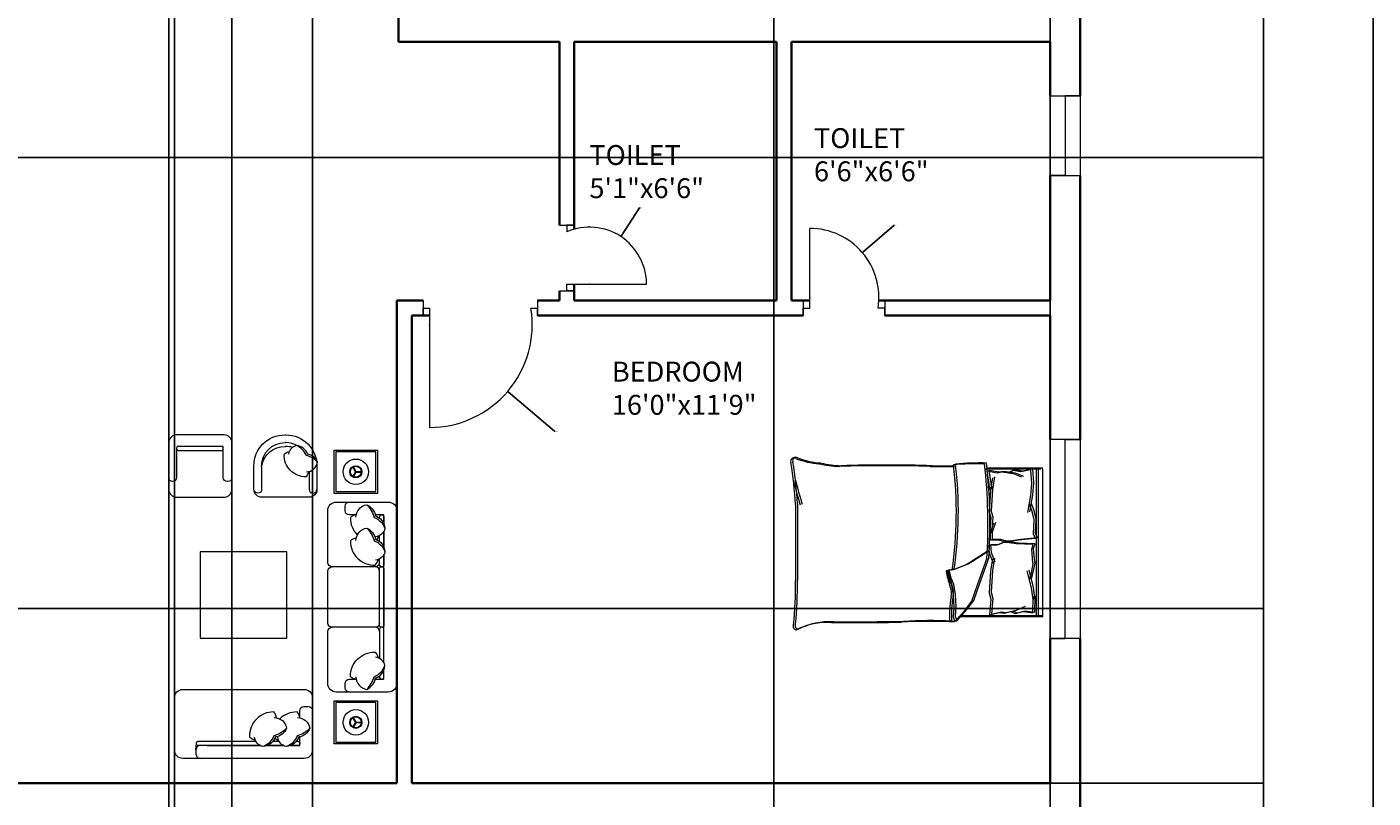
# Model space of a CAD drawing. Units: inches. Extents: x 1902 to 2626, y 1199 to 2408.
# Tile 7 of 9: x 2220 to 2626, y 1817 to 2049. Entities that reach past the tile are written whole.
import ezdxf

# ---------------------------------------------------------------- set-up
doc = ezdxf.new("R2010")
doc.units = ezdxf.units.IN
for name, color, linetype, lineweight in [('A-ANNO-DIMS', 2, 'Continuous', 18), ('A-ANNO-TTLB', 7, 'Continuous', 25), ('A-AREA-IDEN', 7, 'Continuous', 18), ('A-DOOR', 31, 'Continuous', 18), ('A-FURN', 8, 'Continuous', 13), ('A-GLAZ', 181, 'Continuous', 18), ('A-WALL', 7, 'Continuous', 35)]:
    doc.layers.add(name, color=color, linetype=linetype, lineweight=lineweight)
doc.styles.get("Standard").update_dxf_attribs({"font": 'arial.ttf'})
doc.dimstyles.get("Standard").update_dxf_attribs({"dimtxt": 0.18, "dimasz": 0.18, "dimexe": 0.18, "dimexo": 0.0625, "dimgap": 0.09, "dimtad": 0, "dimtih": 1, "dimtoh": 1, "dimdec": 4, "dimzin": 0, "dimdsep": 46, "dimtxsty": 'Standard', "dimcen": 0.09, "dimadec": 0, "dimazin": 0, "dimtfac": 1, "dimtdec": 4, "dimtofl": 0, "dimtmove": 0, "dimatfit": 3, "dimfxl": 1, "dimtolj": 1, "dimtzin": 0, "dimarcsym": 0})

# ---------------------------------------------------------------- blocks, each defined once
blk = doc.blocks.new('BED-DOUBLE')
for p, q in [((25.9, 49.37), (22.87, 45.91)), ((25.9, 49.37), (22.87, 45.91)), ((26.5, 49.58), (23.46, 46.12)), ((26.5, 49.58), (23.46, 46.12)), ((27.53, 49.44), (25.9, 49.37, 3.61)), ((27.53, 49.44), (25.9, 49.37, 3.61)), ((26.48, 47.93), (25.9, 49.37)), ((26.48, 47.93), (25.9, 49.37)), ((28.13, 49.66), (26.5, 49.58, 3.61)), ((28.13, 49.66), (26.5, 49.58, 3.61)), ((27.08, 48.15), (26.5, 49.58)), ((27.08, 48.15), (26.5, 49.58)), ((-0.01, 48.09), (0.59, 48.09)), ((-0.01, 48.09), (-0.01, 3.46)), ((-0.01, 47.87), (24.84, 47.87)), ((-0.01, 47.87), (24.84, 47.87)), ((0.59, 48.09), (25.44, 48.09)), ((0.59, 48.09), (25.44, 48.09)), ((1.43, 3.25), (1.43, 47.87)), ((1.43, 3.25), (1.43, 47.87)), ((2.02, 3.46), (2.02, 48.09)), ((2.02, 3.46), (2.02, 48.09)), ((2.38, 46.8), (2.29, 41.75)), ((2.38, 46.8), (2.29, 41.75)), ((2.38, 46.8), (5.38, 46.44)), ((2.38, 46.8), (5.38, 46.44)), ((2.98, 47.01), (2.89, 41.97)), ((2.98, 47.01), (2.89, 41.96)), ((2.98, 47.01), (5.98, 46.66)), ((2.98, 47.01), (5.98, 46.66)), ((7.7, 46.05), (5.2, 44.94)), ((7.7, 46.05), (5.2, 44.94)), ((5.38, 46.44), (7.78, 47)), ((5.38, 46.44), (7.78, 47)), ((8.3, 46.26), (5.8, 45.16)), ((8.3, 46.26), (5.8, 45.16)), ((5.98, 46.66), (8.38, 47.21)), ((5.98, 46.66), (8.38, 47.21)), ((11.04, 46.8), (7.7, 46.05)), ((11.04, 46.8), (7.7, 46.05)), ((7.78, 47), (8.76, 46.52)), ((7.78, 47), (8.76, 46.52)), ((11.64, 47.01), (8.3, 46.26)), ((11.64, 47.01), (8.3, 46.26)), ((8.38, 47.21), (9.35, 46.73)), ((8.38, 47.21), (9.35, 46.73)), ((12.54, 46.62), (11.04, 46.8)), ((12.54, 46.62), (11.04, 46.8)), ((13.14, 46.83), (11.64, 47.01)), ((13.14, 46.83), (11.64, 47.01)), ((15.47, 47.34), (12.54, 46.62)), ((15.47, 47.34), (12.54, 46.62)), ((16.07, 47.56), (13.14, 46.83)), ((16.07, 47.56), (13.14, 46.83)), ((15.09, 42.55), (15.47, 47.34)), ((15.09, 42.55), (15.47, 47.34)), ((15.69, 42.77), (16.07, 47.56)), ((15.69, 42.77), (16.07, 47.56)), ((22.87, 45.91), (20.84, 43.16)), ((22.87, 45.91), (20.84, 43.16)), ((23.46, 46.12), (21.44, 43.38)), ((23.46, 46.12), (21.44, 43.38)), ((26.19, 45.04), (26.48, 47.93)), ((26.19, 45.04), (26.48, 47.93)), ((26.48, 41.43), (26.19, 45.04)), ((26.48, 41.43), (26.19, 45.04)), ((26.79, 45.26), (27.08, 48.15)), ((26.79, 45.25), (27.08, 48.15)), ((27.08, 41.64), (26.79, 45.26)), ((27.08, 41.64), (26.79, 45.25)), ((2.29, 41.75), (2.37, 42.69)), ((2.29, 41.75), (2.37, 42.69)), ((2.37, 42.69), (2.86, 39.14)), ((2.37, 42.69), (2.86, 39.14)), ((2.89, 41.97), (2.97, 42.9)), ((2.89, 41.96), (2.97, 42.9)), ((2.97, 42.9), (3.46, 39.36)), ((2.97, 42.9), (3.46, 39.35)), ((15.61, 40.72), (15.09, 42.55)), ((15.61, 40.72), (15.09, 42.55)), ((15.21, 34.18), (15.61, 40.72)), ((15.21, 34.18), (15.61, 40.72)), ((16.21, 40.93), (15.69, 42.77)), ((16.21, 40.93), (15.69, 42.77)), ((15.81, 34.39), (16.21, 40.93)), ((15.81, 34.39), (16.21, 40.93)), ((20.84, 43.16), (18.97, 37.96)), ((20.84, 43.16), (18.97, 37.96)), ((21.44, 43.38), (19.56, 38.17)), ((21.44, 43.38), (19.56, 38.17)), ((26.91, 38.25), (26.48, 41.43)), ((26.91, 38.24), (26.48, 41.43)), ((27.51, 38.46), (27.08, 41.64)), ((27.51, 38.46), (27.08, 41.64)), ((2.86, 39.14), (4.12, 34.08)), ((2.86, 39.14), (4.12, 34.08)), ((3.42, 36.61), (2.87, 34.68)), ((3.42, 36.61), (2.87, 34.68)), ((3.46, 39.36), (4.72, 34.29)), ((3.46, 39.35), (4.72, 34.29)), ((4.02, 36.82), (3.47, 34.89)), ((4.02, 36.82), (3.47, 34.89)), ((18.97, 37.96), (16.23, 30.17)), ((18.97, 37.96), (16.23, 30.17)), ((19.56, 38.17), (16.82, 30.38)), ((19.56, 38.17), (16.82, 30.38)), ((27.78, 36.37), (26.91, 38.25)), ((27.78, 36.36), (26.91, 38.24)), ((28.38, 36.58), (27.51, 38.46)), ((28.38, 36.58), (27.51, 38.46)), ((28.96, 34.26), (28.38, 36.58)), ((28.96, 34.26), (28.38, 36.58)), ((73.99, 14.07), (73.99, 37.05)), ((73.99, 14.07), (73.99, 37.05)), ((74.59, 14.28), (74.59, 37.27)), ((74.59, 14.28), (74.59, 37.27)), ((2.87, 34.68), (2.36, 31.94)), ((2.87, 34.68), (2.36, 31.94)), ((3.47, 34.89), (2.96, 32.16)), ((3.47, 34.89), (2.96, 32.16)), ((14.59, 30.41), (15.21, 34.18)), ((14.59, 30.41), (15.21, 34.18)), ((15.18, 30.62), (15.81, 34.39)), ((15.18, 30.62), (15.81, 34.39)), ((22.29, 32.17), (26.48, 33.76)), ((22.29, 32.17), (26.48, 33.76)), ((22.89, 32.38), (27.08, 33.98)), ((22.89, 32.38), (27.08, 33.98)), ((26.48, 33.76), (28.36, 34.05)), ((26.48, 33.76), (28.36, 34.05)), ((27.08, 33.98), (28.96, 34.26)), ((27.08, 33.98), (28.96, 34.26)), ((28.36, 34.05), (27.78, 36.37)), ((28.36, 34.05), (27.78, 36.36)), ((2.36, 31.94), (2.38, 31.64)), ((2.36, 31.94), (2.38, 31.64)), ((2.38, 31.64), (2.78, 27.51)), ((2.38, 31.64), (2.78, 27.51)), ((2.96, 32.16), (2.98, 31.86)), ((2.96, 32.16), (2.98, 31.86)), ((2.98, 31.86), (3.37, 27.72)), ((2.98, 31.86), (3.37, 27.72)), ((15.63, 28.72), (14.43, 31.58)), ((15.63, 28.72), (14.43, 31.58)), ((16.22, 28.93), (15.02, 31.8)), ((16.22, 28.93), (15.02, 31.8)), ((15.77, 26.43), (15.63, 28.72)), ((15.77, 26.43), (15.63, 28.72)), ((16.37, 26.64), (16.22, 28.93)), ((16.37, 26.64), (16.22, 28.93)), ((16.23, 28.26), (22.29, 32.17)), ((16.23, 28.26), (22.29, 32.17)), ((16.82, 28.47), (22.89, 32.38)), ((16.82, 28.47), (22.89, 32.38)), ((1.74, 24.27), (6.74, 24.81)), ((1.74, 24.27), (6.74, 24.81)), ((2.78, 27.51), (2.32, 26.13)), ((2.78, 27.51), (2.32, 26.13)), ((2.32, 26.13), (7.34, 25.9)), ((2.32, 26.13), (7.34, 25.9)), ((2.34, 24.48), (7.33, 25.02)), ((2.34, 24.48), (7.33, 25.02)), ((2.88, 23.13), (2.34, 24.48)), ((2.88, 23.13), (2.34, 24.48)), ((3.37, 27.72), (2.92, 26.34)), ((3.37, 27.72), (2.92, 26.34)), ((2.92, 26.34), (7.94, 26.11)), ((2.92, 26.34), (7.94, 26.11)), ((6.74, 24.81), (9.71, 25.35)), ((6.74, 24.81), (9.71, 25.35)), ((7.33, 25.02), (10.3, 25.56)), ((7.33, 25.02), (10.3, 25.56)), ((7.34, 25.9), (10.34, 25.55)), ((7.34, 25.9), (10.34, 25.55)), ((7.94, 26.11), (10.94, 25.76)), ((7.94, 26.11), (10.94, 25.76)), ((9.71, 25.35), (10.92, 25.35)), ((9.71, 25.35), (10.92, 25.35)), ((10.3, 25.56), (11.52, 25.56)), ((10.3, 25.56), (11.52, 25.56)), ((10.34, 25.55), (11.55, 25.62)), ((10.34, 25.55), (11.55, 25.62)), ((10.92, 25.35), (12.68, 24.81)), ((10.92, 25.35), (12.68, 24.81)), ((10.94, 25.76), (12.15, 25.84)), ((10.94, 25.76), (12.15, 25.84)), ((11.52, 25.56), (13.27, 25.02)), ((11.52, 25.56), (13.27, 25.02)), ((11.55, 25.62), (13.27, 26.27)), ((11.55, 25.62), (13.27, 26.27)), ((12.15, 25.84), (13.87, 26.48)), ((12.15, 25.84), (13.87, 26.48)), ((12.68, 24.81), (15.18, 24.81)), ((12.68, 24.81), (15.18, 24.81)), ((13.27, 26.27), (15.77, 26.43)), ((13.27, 26.27), (15.77, 26.43)), ((13.27, 25.02), (15.78, 25.02)), ((13.27, 25.02), (15.78, 25.02)), ((13.87, 26.48), (16.37, 26.64)), ((13.87, 26.48), (16.37, 26.64)), ((15.18, 24.81), (15.18, 22.51)), ((15.18, 24.81), (15.18, 22.51)), ((15.78, 25.02), (15.78, 22.72)), ((15.78, 25.02), (15.78, 22.72)), ((2.28, 22.92), (1.74, 24.27)), ((2.28, 22.92), (1.74, 24.27)), ((2.15, 18.76), (2.28, 22.92)), ((2.15, 18.76), (2.28, 22.92)), ((2.74, 18.98), (2.88, 23.13)), ((2.74, 18.98), (2.88, 23.13)), ((15.18, 22.51), (14.16, 19.57)), ((15.18, 22.51), (14.16, 19.57)), ((15.78, 22.72), (14.76, 19.79)), ((15.78, 22.72), (14.76, 19.79)), ((15.09, 18.1), (15.47, 22.9)), ((15.09, 18.1), (15.47, 22.9)), ((15.69, 18.32), (16.07, 23.11)), ((15.69, 18.32), (16.07, 23.11)), ((2.15, 18.46), (2.15, 18.76)), ((2.15, 18.46), (2.15, 18.76)), ((2.82, 15.76), (2.15, 18.46)), ((2.82, 15.76), (2.15, 18.46)), ((2.74, 18.68), (2.74, 18.98)), ((2.74, 18.68), (2.74, 18.98)), ((3.42, 15.98), (2.74, 18.68)), ((3.42, 15.98), (2.74, 18.68)), ((3.09, 11.31), (4.04, 16.44)), ((3.09, 11.31), (4.04, 16.44)), ((3.69, 11.52), (4.63, 16.65)), ((3.69, 11.52), (4.63, 16.65)), ((15.61, 16.27), (15.09, 18.1)), ((15.61, 16.27), (15.09, 18.1)), ((15.21, 9.73), (15.61, 16.27)), ((15.21, 9.73), (15.61, 16.27)), ((16.21, 16.49), (15.69, 18.32)), ((16.21, 16.49), (15.69, 18.32)), ((15.81, 9.94), (16.21, 16.49)), ((15.81, 9.94), (16.21, 16.49)), ((3.5, 13.88), (2.82, 15.76)), ((3.5, 13.87), (2.82, 15.76)), ((4.09, 14.09), (3.42, 15.98)), ((4.09, 14.09), (3.42, 15.98)), ((2.82, 7.74), (3.09, 11.31)), ((2.82, 7.74), (3.09, 11.31)), ((3.42, 7.95), (3.69, 11.52)), ((3.42, 7.95), (3.69, 11.52)), ((14.59, 5.96), (15.21, 9.73)), ((14.59, 5.96), (15.21, 9.73)), ((15.18, 6.18), (15.81, 9.94)), ((15.18, 6.18), (15.81, 9.94)), ((15.21, 9.73), (15.51, 8.67)), ((15.21, 9.73), (15.51, 8.67)), ((15.51, 8.67), (16.19, 3.91)), ((15.51, 8.67), (16.19, 3.91)), ((15.81, 9.94), (16.11, 8.88)), ((15.81, 9.94), (16.11, 8.88)), ((16.11, 8.88), (16.78, 4.12)), ((16.11, 8.88), (16.78, 4.12)), ((2.8, 7.64), (2.82, 7.74)), ((2.8, 7.64), (2.82, 7.74)), ((3.11, 3.64), (2.8, 7.64)), ((3.11, 3.64), (2.8, 7.64)), ((3.09, 3.64), (6.06, 4.18)), ((3.09, 3.64), (6.06, 4.18)), ((3.4, 7.86), (3.42, 7.95)), ((3.4, 7.86), (3.42, 7.95)), ((3.71, 3.86), (3.4, 7.86)), ((3.71, 3.86), (3.4, 7.86)), ((3.69, 3.85), (6.66, 4.39)), ((3.69, 3.85), (6.66, 4.39)), ((8.36, 4.72), (5.79, 5.67)), ((8.36, 4.72), (5.79, 5.67)), ((6.06, 4.18), (8.49, 3.78)), ((6.06, 4.18), (8.49, 3.78)), ((8.95, 4.93), (6.39, 5.88)), ((8.95, 4.93), (6.39, 5.88)), ((6.66, 4.39), (9.09, 3.99)), ((6.66, 4.39), (9.09, 3.99)), ((11.73, 4.18), (8.36, 4.72)), ((11.73, 4.18), (8.36, 4.72)), ((8.49, 3.78), (9.44, 4.32)), ((8.49, 3.78), (9.44, 4.32)), ((12.33, 4.39), (8.95, 4.93)), ((12.33, 4.39), (8.95, 4.93)), ((9.09, 3.99), (10.03, 4.53)), ((9.09, 3.99), (10.03, 4.53)), ((13.22, 4.45), (11.73, 4.18)), ((13.22, 4.45), (11.73, 4.18)), ((13.81, 4.66), (12.33, 4.39)), ((13.81, 4.66), (12.33, 4.39)), ((16.19, 3.91), (13.22, 4.45)), ((16.19, 3.91), (13.22, 4.45)), ((16.78, 4.12), (13.81, 4.66)), ((16.78, 4.12), (13.81, 4.66)), ((16.91, 3.25), (-0.01, 3.25)), ((16.91, 3.25), (-0.01, 3.25)), ((17.5, 3.46), (0.59, 3.46)), ((17.5, 3.46), (0.59, 3.46))]:
    blk.add_line(p, q)
for centre, radius, start, end in [((-6.22, 47.93), 33.79, 349.8763, 2.5657), ((-6.22, 47.93), 33.79, 349.8763, 2.5657), ((33.9, 170.19), 120.92, 266.9791, 273.8365), ((33.9, 170.19), 120.92, 266.9791, 273.8365), ((-5.62, 48.14), 33.79, 349.8763, 2.5657), ((-5.62, 48.14), 33.79, 349.8763, 2.5657), ((34.5, 170.41), 120.92, 266.9791, 273.8365), ((34.5, 170.41), 120.92, 266.9791, 273.8365), ((63.32, -4210.02), 4259.62, 90.00217, 90.28689), ((63.32, -4210.02), 4259.62, 90.00217, 90.28689), ((63.92, -4209.8), 4259.62, 90.00217, 90.28689), ((63.92, -4209.8), 4259.62, 90.00217, 90.28689), ((64.11, 71.12), 21.54, 267.4714, 296.4681), ((64.11, 71.12), 21.54, 267.4714, 296.4681), ((64.71, 71.33), 21.54, 267.4714, 296.4681), ((64.71, 71.33), 21.54, 267.4714, 296.4681), ((73.64, 50.81), 1.03, 332.6588, 86.02), ((73.64, 50.81), 1.03, 332.6588, 86.02), ((198.21, 38.43), 124.23, 174.4998, 180.6351), ((198.21, 38.43), 124.23, 174.4998, 180.6351), ((74.24, 51.02), 1.03, 332.6588, 86.02), ((74.24, 51.02), 1.03, 332.6588, 86.02), ((198.8, 38.64), 124.23, 174.4998, 180.6351), ((198.8, 38.64), 124.23, 174.4998, 180.6351), ((32.74, 40.85), 5.81, 168.6608, 203.7384), ((32.74, 40.85), 5.81, 168.6608, 203.7384), ((33.33, 41.06), 5.81, 168.6608, 203.7384), ((33.33, 41.06), 5.81, 168.6608, 203.7384), ((1.38, 29.09), 27.69, 10.6617, 19.8806), ((1.38, 29.09), 27.69, 10.6617, 19.8806), ((1.98, 29.31), 27.69, 10.6617, 19.8806), ((1.98, 29.31), 27.69, 10.6617, 19.8806), ((145.95, 16.58), 120.47, 171.7845, 186.9006), ((145.95, 16.58), 120.47, 171.7845, 186.9006), ((146.55, 16.8), 120.47, 171.7845, 186.9006), ((146.55, 16.8), 120.47, 171.7845, 186.9006), ((28.42, 34.21), 0.172, 250.2464, 1.1377), ((28.42, 34.21), 0.172, 250.2464, 1.1377), ((29.01, 34.43), 0.172, 250.2464, 1.1377), ((29.01, 34.43), 0.172, 250.2464, 1.1377), ((169.99, 19.95), 154.04, 176.0865, 186.7821), ((169.99, 19.95), 154.04, 176.0865, 186.7821), ((170.58, 20.16), 154.04, 176.0865, 186.7821), ((170.58, 20.16), 154.04, 176.0865, 186.7821), ((-22.15, -16.08), 99.41, 13.3832, 17.7053), ((-22.15, -16.08), 99.41, 13.3832, 17.7053), ((-21.55, -15.86), 99.41, 13.3832, 17.7053), ((-21.55, -15.86), 99.41, 13.3832, 17.7053), ((187.53, 20.01), 113.69, 182.9958, 189.4091), ((187.53, 20.01), 113.69, 182.9958, 189.4091), ((188.12, 20.22), 113.69, 182.9958, 189.4091), ((188.12, 20.22), 113.69, 182.9958, 189.4091), ((18.76, 79.52), 77.79, 268.7218, 275.604), ((18.76, 79.52), 77.79, 268.7218, 275.604), ((19.36, 79.74), 77.79, 268.7218, 275.604), ((19.36, 79.74), 77.79, 268.7218, 275.604), ((29.1, -156.22), 158.84, 88.4762, 91.0082), ((29.1, -156.22), 158.84, 88.4762, 91.0082), ((29.7, -156), 158.84, 88.4762, 91.0082), ((29.7, -156.01), 158.84, 88.4762, 91.0082), ((47.26, 452.71), 450.36, 268.2277, 271.7185), ((47.26, 452.71), 450.36, 268.2277, 271.7185), ((47.85, 452.92), 450.36, 268.2277, 271.7185), ((47.85, 452.92), 450.36, 268.2277, 271.7185), ((60.24, -25.11), 27.67, 76.0648, 88.9113), ((60.24, -25.11), 27.67, 76.0648, 88.9113), ((60.83, -24.9), 27.67, 76.0648, 88.9113), ((60.83, -24.9), 27.67, 76.0648, 88.9113), ((65.61, -20.22), 22, 67.9751, 86.652), ((65.61, -20.22), 22, 67.9751, 86.652), ((66.21, -20.01), 22, 67.9751, 86.652), ((66.21, -20.01), 22, 67.9751, 86.652), ((74.43, 1.02), 1.02, 236.1736, 23.4781), ((74.43, 1.02), 1.02, 236.1736, 23.4781), ((75.03, 1.23), 1.02, 236.1736, 23.4781), ((75.03, 1.23), 1.02, 236.1736, 23.4781)]:
    blk.add_arc(centre, radius, start, end)
blk = doc.blocks.new('WINDOW-60-A')
for p, q in [((0, 9), (0, 0)), ((60, 9), (0, 9)), ((60, 4.5), (60, 9)), ((60, 9), (60, 0)), ((0, 0), (0, 4.5)), ((0, 4.5), (60, 4.5)), ((0, 0), (60, 0))]:
    blk.add_line(p, q)
blk = doc.blocks.new('WINDOW-24')
for p, q in [((0, 24), (9, 24)), ((0, 24), (0, 0)), ((9, 24), (4.5, 24)), ((4.5, 24), (4.5, 0)), ((9, 24), (9, 0)), ((4.5, 0), (0, 0)), ((0, 0), (9, 0))]:
    blk.add_line(p, q)
blk = doc.blocks.new('TABLE-END-WITH-LAMP')
for p, q in [((6.59, 6.55), (5.67, 8.14)), ((6.45, 6.47), (5.53, 8.06)), ((6.45, 6.55), (5.53, 4.96)), ((6.59, 6.47), (5.67, 4.88)), ((6.52, 6.59), (8.35, 6.59)), ((6.52, 6.43), (8.35, 6.43))]:
    blk.add_line(p, q)
at = {"ltscale": 0.03}
blk.add_lwpolyline([(0.01, 0), (0.01, 13.02), (13.03, 13.02), (13.03, 0)], close=True, dxfattribs=at)
blk.add_lwpolyline([(0.53, 12.5), (0.53, 0.52), (12.51, 0.52), (12.51, 12.5)], close=True)
for radius in [3.84, 1.84, 1.65]:
    blk.add_circle((6.52, 6.51), radius)
blk = doc.blocks.new('TABLE-COFFEE-SQUARE')
at = {"ltscale": 0.03}
blk.add_lwpolyline([(0, 26.05), (0, 0), (26.05, 0), (26.05, 26.05)], close=True, dxfattribs=at)
blk = doc.blocks.new('*D33')
at = {"layer": 'A-ANNO-DIMS', "color": 0, "lineweight": -2, "transparency": 16777216}
for p, q in [((2537.91, 2289.47), (2593.33, 2289.47)), ((2593.15, 2289.29), (2593.15, 2055.66)), ((2593.15, 1821.65), (2593.15, 2055.29)), ((2528.91, 1821.47), (2593.33, 1821.47))]:
    blk.add_line(p, q, dxfattribs=at)
at = {"layer": 'A-ANNO-DIMS', "color": 0, "transparency": 16777216}
for points in [[(2593.12, 2289.29), (2593.18, 2289.29), (2593.15, 2289.47)], [(2593.12, 1821.65), (2593.18, 1821.65), (2593.15, 1821.47)]]:
    blk.add_solid(points, dxfattribs=at)
at = {"layer": 'Defpoints', "color": 0, "transparency": 16777216}
for p in [(2537.85, 2289.47), (2593.15, 2289.47), (2528.85, 1821.47)]:
    blk.add_point(p, dxfattribs=at)
at = {"layer": 'A-ANNO-DIMS', "color": 0, "transparency": 16777216, "insert": (2593.15, 2055.47), "char_height": 0.18, "attachment_point": 5}
blk.add_mtext('\\A1;468', dxfattribs=at)
blk = doc.blocks.new('*D34')
at = {"layer": 'A-ANNO-DIMS', "color": 0, "lineweight": -2, "transparency": 16777216}
for p, q in [((2528.91, 1821.47), (2593.33, 1821.47)), ((2593.15, 1821.29), (2593.15, 1613.15)), ((2593.15, 1404.65), (2593.15, 1612.79)), ((2537.91, 1404.47), (2593.33, 1404.47))]:
    blk.add_line(p, q, dxfattribs=at)
at = {"layer": 'A-ANNO-DIMS', "color": 0, "transparency": 16777216}
for points in [[(2593.12, 1821.29), (2593.18, 1821.29), (2593.15, 1821.47)], [(2593.12, 1404.65), (2593.18, 1404.65), (2593.15, 1404.47)]]:
    blk.add_solid(points, dxfattribs=at)
at = {"layer": 'Defpoints', "color": 0, "transparency": 16777216}
for p in [(2528.85, 1821.47), (2593.15, 1821.47), (2537.85, 1404.47)]:
    blk.add_point(p, dxfattribs=at)
at = {"layer": 'A-ANNO-DIMS', "color": 0, "transparency": 16777216, "insert": (2593.15, 1612.97), "char_height": 0.18, "attachment_point": 5}
blk.add_mtext('\\A1;417', dxfattribs=at)
blk = doc.blocks.new('*D37')
at = {"layer": 'A-ANNO-DIMS', "color": 0, "lineweight": -2, "transparency": 16777216}
for p, q in [((2445.52, 2280.41), (2445.52, 1198.67)), ((2528.85, 2280.41), (2528.85, 1198.67)), ((2445.7, 1198.85), (2486.79, 1198.85)), ((2528.67, 1198.85), (2487.58, 1198.85))]:
    blk.add_line(p, q, dxfattribs=at)
at = {"layer": 'A-ANNO-DIMS', "color": 0, "transparency": 16777216}
for points in [[(2445.7, 1198.88), (2445.7, 1198.82), (2445.52, 1198.85)], [(2528.67, 1198.88), (2528.67, 1198.82), (2528.85, 1198.85)]]:
    blk.add_solid(points, dxfattribs=at)
at = {"layer": 'Defpoints', "color": 0, "transparency": 16777216}
for p in [(2445.52, 2280.47), (2528.85, 2280.47), (2528.85, 1198.85)]:
    blk.add_point(p, dxfattribs=at)
at = {"layer": 'A-ANNO-DIMS', "color": 0, "transparency": 16777216, "insert": (2487.18, 1198.85), "char_height": 0.18, "attachment_point": 5}
blk.add_mtext('\\A1;83.33', dxfattribs=at)
blk = doc.blocks.new('*D39')
at = {"layer": 'A-ANNO-DIMS', "color": 0, "lineweight": -2, "transparency": 16777216}
for p, q in [((2128.41, 2010.11), (2593.33, 2010.11)), ((2593.15, 2009.93), (2593.15, 1942.29)), ((2593.15, 1874.29), (2593.15, 1941.93)), ((2128.41, 1874.11), (2593.33, 1874.11))]:
    blk.add_line(p, q, dxfattribs=at)
at = {"layer": 'A-ANNO-DIMS', "color": 0, "transparency": 16777216}
for points in [[(2593.12, 2009.93), (2593.18, 2009.93), (2593.15, 2010.11)], [(2593.12, 1874.29), (2593.18, 1874.29), (2593.15, 1874.11)]]:
    blk.add_solid(points, dxfattribs=at)
at = {"layer": 'Defpoints', "color": 0, "transparency": 16777216}
for p in [(2128.35, 2010.11), (2593.15, 2010.11), (2128.35, 1874.11)]:
    blk.add_point(p, dxfattribs=at)
at = {"layer": 'A-ANNO-DIMS', "color": 0, "transparency": 16777216, "insert": (2593.15, 1942.11), "char_height": 0.18, "attachment_point": 5}
blk.add_mtext('\\A1;136', dxfattribs=at)
blk = doc.blocks.new('*D41')
at = {"layer": 'A-ANNO-DIMS', "color": 0, "lineweight": -2, "transparency": 16777216}
for p, q in [((2264.77, 1723.47), (2264.77, 2377.95)), ((2264.95, 2377.77), (2285.22, 2377.77)), ((2306.27, 2377.77), (2286.01, 2377.77)), ((2306.45, 1723.47), (2306.45, 2377.95))]:
    blk.add_line(p, q, dxfattribs=at)
at = {"layer": 'A-ANNO-DIMS', "color": 0, "transparency": 16777216}
for points in [[(2264.95, 2377.8), (2264.95, 2377.74), (2264.77, 2377.77)], [(2306.27, 2377.8), (2306.27, 2377.74), (2306.45, 2377.77)]]:
    blk.add_solid(points, dxfattribs=at)
at = {"layer": 'Defpoints', "color": 0, "transparency": 16777216}
for p in [(2306.45, 2377.77), (2264.77, 1723.41), (2306.45, 1723.41)]:
    blk.add_point(p, dxfattribs=at)
at = {"layer": 'A-ANNO-DIMS', "color": 0, "transparency": 16777216, "insert": (2285.61, 2377.77), "char_height": 0.18, "attachment_point": 5}
blk.add_mtext('\\A1;41.68', dxfattribs=at)
blk = doc.blocks.new('*D43')
at = {"layer": 'A-ANNO-DIMS', "color": 0, "lineweight": -2, "transparency": 16777216}
for p, q in [((2263.07, 1800.47), (2263.07, 2377.95)), ((2263.25, 2377.77), (2272.13, 2377.77)), ((2281.92, 2377.77), (2273.04, 2377.77)), ((2282.1, 1800.47), (2282.1, 2377.95))]:
    blk.add_line(p, q, dxfattribs=at)
at = {"layer": 'A-ANNO-DIMS', "color": 0, "transparency": 16777216}
for points in [[(2263.25, 2377.8), (2263.25, 2377.74), (2263.07, 2377.77)], [(2281.92, 2377.8), (2281.92, 2377.74), (2282.1, 2377.77)]]:
    blk.add_solid(points, dxfattribs=at)
at = {"layer": 'Defpoints', "color": 0, "transparency": 16777216}
for p in [(2282.1, 2377.77), (2263.07, 1800.41), (2282.1, 1800.41)]:
    blk.add_point(p, dxfattribs=at)
at = {"layer": 'A-ANNO-DIMS', "color": 0, "transparency": 16777216, "insert": (2272.58, 2377.77), "char_height": 0.18, "attachment_point": 5}
blk.add_mtext('\\A1;19.024', dxfattribs=at)
blk = doc.blocks.new('*D45')
at = {"layer": 'A-ANNO-DIMS', "color": 0, "lineweight": -2, "transparency": 16777216}
for p, q in [((2341.64, 1959.66), (2341.82, 1959.66)), ((2341.73, 1959.57), (2341.73, 1959.75)), ((2379.41, 1927.56), (2365.42, 1939.48)), ((2379.59, 1927.56), (2379.41, 1927.56))]:
    blk.add_line(p, q, dxfattribs=at)
at = {"layer": 'A-ANNO-DIMS', "color": 0, "transparency": 16777216}
blk.add_solid([(2365.44, 1939.51), (2365.4, 1939.46), (2365.28, 1939.6)], dxfattribs=at)
at = {"layer": 'Defpoints', "color": 0, "transparency": 16777216}
for p in [(2341.73, 1959.66), (2365.28, 1939.6)]:
    blk.add_point(p, dxfattribs=at)
at = {"layer": 'A-ANNO-DIMS', "color": 0, "transparency": 16777216, "insert": (2380.07, 1927.56), "char_height": 0.18, "attachment_point": 5}
blk.add_mtext('\\A1;R30.94', dxfattribs=at)
blk = doc.blocks.new('*D55')
at = {"layer": 'A-ANNO-DIMS', "color": 0, "lineweight": -2, "transparency": 16777216}
for p, q in [((2481.65, 1989.57), (2472.31, 1981.57)), ((2481.83, 1989.57), (2481.65, 1989.57)), ((2456.28, 1967.92), (2456.46, 1967.92)), ((2456.37, 1967.83), (2456.37, 1968.01))]:
    blk.add_line(p, q, dxfattribs=at)
at = {"layer": 'A-ANNO-DIMS', "color": 0, "transparency": 16777216}
blk.add_solid([(2472.29, 1981.59), (2472.33, 1981.55), (2472.17, 1981.45)], dxfattribs=at)
at = {"layer": 'Defpoints', "color": 0, "transparency": 16777216}
for p in [(2472.17, 1981.45), (2456.37, 1967.92)]:
    blk.add_point(p, dxfattribs=at)
at = {"layer": 'A-ANNO-DIMS', "color": 0, "transparency": 16777216, "insert": (2482.24, 1989.57), "char_height": 0.18, "attachment_point": 5}
blk.add_mtext('\\A1;R20.8', dxfattribs=at)
blk = doc.blocks.new('*D60')
at = {"layer": 'A-ANNO-DIMS', "color": 0, "lineweight": -2, "transparency": 16777216}
for p, q in [((2405, 1994.89), (2399.45, 1986.43)), ((2405.18, 1994.89), (2405, 1994.89)), ((2389.85, 1971.93), (2390.03, 1971.93)), ((2389.94, 1971.84), (2389.94, 1972.02))]:
    blk.add_line(p, q, dxfattribs=at)
at = {"layer": 'A-ANNO-DIMS', "color": 0, "transparency": 16777216}
blk.add_solid([(2399.42, 1986.45), (2399.47, 1986.41), (2399.35, 1986.28)], dxfattribs=at)
at = {"layer": 'Defpoints', "color": 0, "transparency": 16777216}
for p in [(2399.35, 1986.28), (2389.94, 1971.93)]:
    blk.add_point(p, dxfattribs=at)
at = {"layer": 'A-ANNO-DIMS', "color": 0, "transparency": 16777216, "insert": (2405.73, 1994.89), "char_height": 0.18, "attachment_point": 5}
blk.add_mtext('\\A1;R17.163', dxfattribs=at)

msp = doc.modelspace()

# ---------------------------------------------------------------- linework, layer by layer
at = {"layer": 'A-ANNO-TTLB'}
msp.add_lwpolyline([(1901.6928, 2408.1473), (2626.1646, 2408.1473), (2626.1646, 1206.3103), (1901.6928, 1206.3103)], close=True, dxfattribs=at)
at = {"layer": 'A-DOOR'}
for p, q in [((2380.8507, 1989.6712), (2385.3507, 1989.6712)), ((2385.3507, 1989.6712), (2383.1007, 1989.6712)), ((2383.1007, 1989.6712), (2383.1007, 1987.6712)), ((2456.3714, 1964.7233), (2456.3714, 1988.7233)), ((2380.8507, 1969.9292), (2385.3507, 1969.9292)), ((2383.1007, 1969.9292), (2383.1007, 1971.9292)), ((2383.1007, 1971.9292), (2407.1007, 1971.9292)), ((2385.3507, 1969.9292), (2383.1007, 1969.9292)), ((2339.7263, 1966.9733), (2339.7263, 1962.4733)), ((2339.7263, 1962.4733), (2339.7263, 1964.7233)), ((2339.7263, 1964.7233), (2341.7263, 1964.7233)), ((2341.7263, 1964.7233), (2341.7263, 1940.7233)), ((2374.2725, 1964.5854), (2372.2725, 1964.5854)), ((2374.2725, 1966.9733), (2374.2725, 1963.4615)), ((2374.2725, 1962.4733), (2374.2725, 1964.5854)), ((2454.3714, 1966.9733), (2454.3714, 1962.4733)), ((2454.3714, 1962.4733), (2454.3714, 1964.7233)), ((2454.3714, 1964.7233), (2454.3714, 1964.7233)), ((2454.3714, 1964.7233), (2456.3714, 1964.7233)), ((2478.9238, 1964.7233), (2476.9238, 1964.7233)), ((2478.9238, 1966.9733), (2478.9238, 1962.4733)), ((2478.9238, 1962.4733), (2478.9238, 1964.7233)), ((2374.2725, 1963.4615), (2374.2725, 1962.4733)), ((2341.7263, 1940.7233), (2341.7263, 1928.7233))]:
    msp.add_line(p, q, dxfattribs=at)
for centre, radius, start, end in [((2389.938, 1971.9292), 17.1627, 360, 113.476935), ((2456.3714, 1967.9233), 20.8, 351.150212, 90), ((2341.7263, 1959.6635), 30.9402, 270, 9.153494)]:
    msp.add_arc(centre, radius, start, end, dxfattribs=at)
at = {"layer": 'A-FURN'}
msp.add_line((2271.2864, 1831.5107), (2271.4129, 1833.4644), dxfattribs=at)
at = {"layer": 'A-FURN', "ltscale": 0.03}
for points in [[(2265.4197, 1926.485), (2265.4197, 1926.485, 0.41421356), (2263.071, 1924.1363), (2263.071, 1910.0441, 0.41421356), (2265.4197, 1907.6955), (2265.4197, 1907.6955), (2279.7467, 1907.6955, 0.41421356), (2282.0954, 1910.0441), (2282.0954, 1924.1363, 0.41421356), (2279.7467, 1926.485)], [(2313.6163, 1848.9269, -0.41421356), (2311.0114, 1851.5318), (2311.0114, 1867.1613, -0.41421356), (2312.3138, 1868.4638, -0.41421356), (2311.0114, 1869.7662), (2311.0114, 1885.3957, -0.41421356), (2312.3138, 1886.6982, -0.41421356), (2311.0114, 1888.0006), (2311.0114, 1903.6301, -0.41421356), (2313.6163, 1906.2351), (2329.2458, 1906.2351, -0.41421356), (2331.8507, 1903.6301), (2331.8507, 1851.5318, -0.41421356), (2329.2458, 1848.9269)], [(2264.7741, 1847.1402, -0.41421356), (2267.379, 1849.7451), (2267.379, 1849.7451, 0.31783725), (2267.379, 1849.7451, -0.41421356), (2267.379, 1849.7451), (2267.379, 1849.7451, 1.18618475), (2267.379, 1849.7451, -0.41421356), (2267.379, 1849.7451), (2303.8478, 1849.7451, -0.41421356), (2306.4528, 1847.1402), (2306.4528, 1831.5107, -0.41421356), (2303.8478, 1828.9058), (2267.379, 1828.9058, -0.41421356), (2264.7741, 1831.5107)]]:
    msp.add_lwpolyline(points, format="xyb", close=True, dxfattribs=at)
msp.add_lwpolyline([(2298.2473, 1907.6955), (2291.0838, 1907.6955, -0.41421356), (2288.7351, 1910.0441), (2288.7351, 1917.0902, -0.41421356), (2298.1298, 1926.485), (2298.2473, 1926.485), (2298.3647, 1926.485, -0.41421356), (2307.7595, 1917.0902), (2307.7595, 1910.0441, -0.41421356), (2305.4108, 1907.6955), (2298.2473, 1907.6955)], format="xyb", dxfattribs=at)
at = {"layer": 'A-FURN'}
for points in [[(2291.0838, 1917.0902, -0.41421356), (2298.1298, 1924.1363), (2298.2473, 1924.1363)], [(2301.8623, 1923.207, 0.13059149), (2298.3647, 1924.1363), (2298.2473, 1924.1363)], [(2265.4197, 1922.2574), (2265.4197, 1913.5672, -0.41421356), (2264.2453, 1912.3928), (2264.2453, 1912.3928, -0.41421356), (2263.071, 1913.5672)], [(2275.0876, 1922.962), (2265.8894, 1922.962, 0.41421356), (2265.4197, 1922.4922), (2265.4197, 1922.2574, 0.41421356), (2265.8894, 1921.7876), (2273.9051, 1921.7876, 0.41421356)], [(2273.9051, 1921.7876), (2279.0421, 1921.7876, 0.41421356), (2279.5118, 1922.2574), (2279.5118, 1922.4922, 0.41421356), (2279.0421, 1922.962)], [(2279.0421, 1922.962), (2275.0876, 1922.962, 0.41421356)], [(2291.0838, 1917.0902, -0.37271891), (2298.1298, 1922.962), (2298.2473, 1922.962)], [(2305.1785, 1915.3872, -0.16554063), (2304.452, 1913.8356, -0.42598917), (2297.8566, 1920.563, -0.12152332), (2299.4222, 1921.4903, 7.11546429)], [(2300.3669, 1922.7089, 0.07238424), (2298.3647, 1922.962), (2298.2473, 1922.962)], [(2304.9935, 1920.4548, 0.30666349), (2301.4908, 1923.254, 0.30632997), (2299.2026, 1920.6976, -0.87284716)], [(2307.9516, 1918.2757, 0.14772988), (2304.5193, 1920.2939, 0.21334276), (2301.4908, 1923.254, 0.17866181)], [(2304.5866, 1915.3156, 0.35677236), (2307.9516, 1918.2757, 0.24954205), (2304.9026, 1920.715, -9.61688035)], [(2291.0838, 1917.0903), (2291.0838, 1910.0441, -0.41421356), (2289.9094, 1908.8698), (2289.9094, 1908.8698, -0.41421356), (2288.7351, 1910.0441)], [(2282.0954, 1913.5672, -0.41421356), (2280.921, 1912.3928), (2280.6862, 1912.3928, -0.41421356), (2279.5118, 1913.5672), (2279.5118, 1915.3867)], [(2305.4108, 1915.4437), (2305.4108, 1910.0441, 0.41421356), (2306.5851, 1908.8698), (2306.5851, 1908.8698, 0.41421356), (2307.7595, 1910.0441)], [(2319.5416, 1902.3277), (2317.5236, 1902.3277, -0.41421356), (2316.2212, 1903.6301), (2316.2212, 1904.9326, -0.41421356), (2317.5236, 1906.2351)], [(2319.4628, 1901.6741, -0.35677236), (2322.7458, 1905.4061, -0.24954205), (2325.4513, 1902.0245)], [(2322.7458, 1905.4061, -0.14772988), (2324.9842, 1901.5994, -0.21334276), (2328.2672, 1898.2406)], [(2319.5422, 1902.3305, 0.16554063), (2317.8213, 1901.5248, 0.20023115), (2319.9172, 1896.3545)], [(2325.1626, 1902.1253, -0.30666349), (2328.2672, 1898.2406, -0.30632997), (2325.4319, 1895.7027)], [(2327.9433, 1899.5877), (2327.9433, 1902.3277), (2325.3837, 1902.3277, -0.41435211)], [(2326.6408, 1901.3338), (2326.6408, 1901.8067, -0.41421356), (2327.1618, 1902.3277), (2327.4223, 1902.3277, -0.41421356), (2327.9433, 1901.8067)], [(2327.9433, 1901.8067), (2327.9433, 1899.5877, -0.41446868)], [(2319.4628, 1894.6578, -0.35677236), (2322.7458, 1898.3898, -0.24954205), (2325.4513, 1895.0082)], [(2322.7458, 1898.3898, -0.14772988), (2324.9842, 1894.5831, -0.21334276), (2328.2672, 1891.2243)], [(2325.8019, 1894.8544, 0.07186538), (2326.3111, 1895.9463)], [(2326.6408, 1894.3175), (2326.6408, 1896.1094, -0.41459885)], [(2327.9433, 1897.4209), (2327.9433, 1892.5714, -0.41474665)], [(2319.5422, 1895.3142, 0.16554063), (2317.8213, 1894.5085, 0.42598917), (2325.2827, 1887.1936, 0.12152332), (2326.3111, 1888.93)], [(2325.1626, 1895.109, -0.30666349), (2328.2672, 1891.2243, -0.30632997), (2325.4319, 1888.6865)], [(2326.6408, 1888.0006, -0.41421356), (2325.3384, 1886.6982), (2312.3138, 1886.6982, -0.41732018)], [(2327.9433, 1890.4046), (2327.9433, 1887.2192, -0.41421356), (2327.4223, 1886.6982), (2327.1618, 1886.6982, -0.41421356), (2326.6408, 1887.2192), (2326.6408, 1889.0931, -0.12631336)], [(2326.6408, 1885.3957, 0.41421356), (2325.3384, 1886.6982)], [(2326.6408, 1867.1613, 0.41421356), (2325.3384, 1868.4638), (2312.3138, 1868.4638, 0.4152491)], [(2326.6408, 1869.7662, -0.41421356), (2325.3384, 1868.4638)], [(2327.9433, 1857.7411), (2327.9433, 1867.9428, 0.41421356), (2327.4223, 1868.4638), (2327.1618, 1868.4638, 0.41421356), (2326.6408, 1867.9428), (2326.6408, 1859.0526, 0.41265155)], [(2319.5422, 1852.8315, -0.16554063), (2317.8213, 1853.6372, -0.42598917), (2325.2827, 1860.9521, -0.12152332), (2326.3111, 1859.2156)], [(2325.1626, 1853.0367, 0.30666349), (2328.2672, 1856.9214, 0.30632997), (2325.4319, 1859.4592)], [(2322.7458, 1849.7558, 0.14772988), (2324.9842, 1853.5626, 0.21334276), (2328.2672, 1856.9214)], [(2327.9433, 1853.3553), (2327.9433, 1855.5743, 0.41253535)], [(2317.5236, 1848.9269, -0.41421356), (2316.2212, 1850.2294), (2316.2212, 1851.5318, -0.41421356), (2317.5236, 1852.8343), (2319.5416, 1852.8343)], [(2319.4628, 1853.4879, 0.35677236), (2322.7458, 1849.7558, 0.24954205), (2325.4513, 1853.1374)], [(2326.6408, 1853.8282), (2326.6408, 1853.3553, 0.41421356), (2327.1618, 1852.8343), (2327.4223, 1852.8343, 0.41421356), (2327.9433, 1853.3553)], [(2295.5319, 1841.2143, 0.16554063), (2294.7262, 1842.9352, 0.42598917), (2287.4113, 1835.4738, 0.12152332), (2289.1477, 1834.4454, -7.11546429)], [(2302.5482, 1841.2143, 0.16554063), (2301.7425, 1842.9352, 0.20023115), (2296.5722, 1840.8393, 0.12152332)], [(2302.5454, 1841.2148), (2302.5454, 1843.2328, -0.41421356), (2303.8478, 1844.5353), (2305.1503, 1844.5353, -0.41421356), (2306.4528, 1843.2328)], [(2294.8755, 1841.2937, -0.35677236), (2298.6075, 1838.0107, -0.24954205), (2295.2259, 1835.3052, 9.61688035)], [(2301.8918, 1841.2937, -0.35677236), (2305.6238, 1838.0107, -0.24954205), (2302.2422, 1835.3052, 9.61688035)], [(2295.3267, 1835.5939, -0.30666349), (2291.442, 1832.4893, -0.30632997), (2288.9042, 1835.3246, 0.87284716)], [(2298.6075, 1838.0107, -0.14772988), (2294.8008, 1835.7723, -0.21334276), (2291.442, 1832.4893, -0.17866181)], [(2295.0721, 1834.9546, 0.07186538), (2296.164, 1834.4454, -7.11546429)], [(2302.343, 1835.5939, -0.30666349), (2298.4583, 1832.4893, -0.30632997), (2295.9204, 1835.3246, 0.87284716)], [(2305.6238, 1838.0107, -0.14772988), (2301.8171, 1835.7723, -0.21334276), (2298.4583, 1832.4893, -0.17866181)], [(2299.8054, 1832.8132), (2302.5454, 1832.8132), (2302.5454, 1835.3728, -0.41421356)], [(2274.6068, 1832.8132), (2272.5889, 1832.8132, 0.41421356), (2271.2864, 1831.5107), (2271.2864, 1830.2083, 0.41421356), (2272.5889, 1828.9058)], [(2290.6223, 1832.8132), (2271.9339, 1832.8132, -0.41421356), (2271.4129, 1833.3341), (2271.4129, 1833.5946, -0.41421356), (2271.9339, 1834.1156), (2289.3108, 1834.1156, -0.41421356)], [(2297.6386, 1832.8132), (2292.7891, 1832.8132, -0.41421356)], [(2294.5352, 1834.1156), (2296.3271, 1834.1156, -0.41421356)], [(2302.0244, 1832.8132), (2299.8054, 1832.8132, -0.41421356)], [(2301.5515, 1834.1156), (2302.0244, 1834.1156, -0.41421356), (2302.5454, 1833.5946), (2302.5454, 1833.3341, -0.41421356), (2302.0244, 1832.8132)]]:
    msp.add_lwpolyline(points, format="xyb", dxfattribs=at)
for points in [[(2275.0876, 1922.962), (2265.5371, 1922.962)], [(2279.5118, 1915.3867), (2279.5118, 1922.962), (2275.0876, 1922.962)], [(2327.9433, 1892.5714), (2327.9433, 1897.4209)], [(2327.9433, 1857.7411), (2327.9433, 1890.4046)], [(2325.3837, 1852.8343), (2327.9433, 1852.8343), (2327.9433, 1855.5743)], [(2274.6068, 1832.8132), (2290.6223, 1832.8132)], [(2292.7891, 1832.8132), (2297.6386, 1832.8132)]]:
    msp.add_lwpolyline(points, dxfattribs=at)
msp.add_lwpolyline([(2327.9433, 1886.1772), (2327.9433, 1868.9848, -0.41421356), (2327.4223, 1868.4638), (2327.1618, 1868.4638, -0.41421356), (2326.6408, 1868.9848), (2326.6408, 1886.1772, -0.41421356), (2327.1618, 1886.6982), (2327.4223, 1886.6982, -0.41421356)], format="xyb", close=True, dxfattribs=at)
at = {"layer": 'A-WALL'}
for p, q in [((2332.3507, 2067.5809), (2332.3507, 2044.9733)), ((2537.8507, 2069.0784), (2537.8507, 2028.722)), ((2380.8507, 2044.9733), (2332.3507, 2044.9733)), ((2380.8507, 2044.9733), (2380.8507, 1989.6712)), ((2385.3507, 2044.9733), (2385.3507, 1988.4675)), ((2446.3507, 2044.9733), (2385.3507, 2044.9733)), ((2446.3507, 2044.9733), (2446.3507, 1966.9733)), ((2528.8507, 2044.9733), (2450.8507, 2044.9733)), ((2450.8507, 2044.9733), (2450.8507, 1966.9733)), ((2528.8507, 2044.9733), (2528.8507, 2028.722)), ((2528.8507, 2004.722), (2528.8507, 1966.9733)), ((2537.8507, 2004.722), (2537.8507, 1925.0569)), ((2380.8507, 1969.9292), (2380.8507, 1966.9733)), ((2385.3507, 1971.9292), (2385.3507, 1966.9733)), ((2331.8507, 1966.9733), (2339.7263, 1966.9733)), ((2331.8507, 1966.9733), (2331.8507, 1821.4733)), ((2374.2725, 1966.9733), (2380.8507, 1966.9733)), ((2385.3507, 1966.9733), (2446.3507, 1966.9733)), ((2450.8507, 1966.9733), (2456.3714, 1966.9733)), ((2477.1497, 1966.9733), (2528.8507, 1966.9733)), ((2336.3507, 1962.4733), (2336.3507, 1821.4733)), ((2341.7263, 1962.4733), (2336.3507, 1962.4733)), ((2454.3714, 1962.4733), (2374.2725, 1962.4733)), ((2528.8507, 1962.4733), (2478.9238, 1962.4733)), ((2528.8507, 1962.4733), (2528.8507, 1925.0569)), ((2528.8507, 1865.0569), (2528.8507, 1821.4733)), ((2537.8507, 1865.0569), (2537.8507, 1754.0445)), ((2331.8507, 1821.4733), (2137.3507, 1821.4733)), ((2528.8507, 1821.4733), (2336.3507, 1821.4733))]:
    msp.add_line(p, q, dxfattribs=at)

# ---------------------------------------------------------------- block references
at = {"layer": 'A-FURN'}
for name, p in [('TABLE-END-WITH-LAMP', (2312.96, 1908.8413)), ('TABLE-COFFEE-SQUARE', (2272.59, 1865.2087)), ('TABLE-END-WITH-LAMP', (2312.96, 1833.2987))]:
    msp.add_blockref(name, p, dxfattribs=at)
at = {"layer": 'A-FURN', "rotation": 180}
msp.add_blockref('BED-DOUBLE', (2526.6052, 1919.7413), dxfattribs=at)
at = {"layer": 'A-GLAZ'}
msp.add_blockref('WINDOW-24', (2528.85, 2004.72), dxfattribs=at)
at = {"layer": 'A-GLAZ', "extrusion": (0, 0, -1), "zscale": -1, "rotation": 90}
msp.add_blockref('WINDOW-60-A', (-2528.8474, 1865.0609), dxfattribs=at)

# ---------------------------------------------------------------- texts
at = {"layer": 'A-AREA-IDEN', "char_height": 6, "attachment_point": 1}
for s, width, insert in [('TOILET\\P6\'6"x6\'6"', 99.286264, (2457.5997, 2018.9426)), ('TOILET\\P5\'1"x6\'6"', 179.962319, (2389.8914, 2013.8535)), ('BEDROOM\\P16\'0"x11\'9"', 169.030384, (2396.6506, 1948.5457))]:
    msp.add_mtext_dynamic_manual_height_columns(s, width=width, gutter_width=12.5, heights=[0], dxfattribs=dict(at, insert=insert))

# ---------------------------------------------------------------- dimensions: what is measured, and where the dimension line sits
at = {"layer": 'A-ANNO-DIMS'}
for base, p1, p2, override, picture, middle in [((2282.0954, 2377.7733), (2263.071, 1800.4076), (2282.0954, 1800.4076), {"dimdec": 3, "dimlfac": 1, "dimrnd": 0, "dimzin": 0, "dimdsep": 46, "dimlunit": 2}, '*D43', (2272.5832, 2377.7733)), ((2306.4528, 2377.7733), (2264.7741, 1723.4115), (2306.4528, 1723.4115), {"dimdec": 2, "dimlfac": 1, "dimrnd": 0, "dimzin": 0, "dimdsep": 46, "dimlunit": 2}, '*D41', (2285.6134, 2377.7733)), ((2528.8507, 1198.8475), (2445.516, 2280.4733), (2528.8507, 2280.4733), {"dimdec": 2, "dimlfac": 1, "dimrnd": 0, "dimzin": 0, "dimdsep": 46, "dimlunit": 2}, '*D37', (2487.1833, 1198.8475))]:
    dim = msp.add_linear_dim(base=base, p1=p1, p2=p2, dimstyle='Standard', override=override, dxfattribs=at)
    dim.commit()
    dim.dimension.update_dxf_attribs({"geometry": picture, "text_midpoint": middle})
for base, p1, p2, picture, middle in [((2593.1507, 2289.4733), (2528.8507, 1821.4733), (2537.8507, 2289.4733), '*D33', (2593.1507, 2055.4733)), ((2593.1507, 2010.11), (2128.3507, 1874.11), (2128.3507, 2010.11), '*D39', (2593.1507, 1942.11)), ((2593.1507, 1821.4733), (2537.8507, 1404.4733), (2528.8507, 1821.4733), '*D34', (2593.1507, 1612.9733))]:
    dim = msp.add_linear_dim(base=base, p1=p1, p2=p2, angle=90, dimstyle='Standard', override={"dimdec": 0, "dimlfac": 1, "dimrnd": 0, "dimzin": 0, "dimdsep": 46, "dimlunit": 2}, dxfattribs=at)
    dim.commit()
    dim.dimension.update_dxf_attribs({"geometry": picture, "text_midpoint": middle})
for center, mpoint, override, picture, middle in [((2389.938, 1971.9292), (2399.3511, 1986.2802), {"dimdec": 3, "dimlfac": 1, "dimrnd": 0, "dimzin": 0, "dimdsep": 46, "dimlunit": 2}, '*D60', (2405.7288, 1994.8908)), ((2456.3714, 1967.9233), (2472.1699, 1981.4529), {"dimdec": 1, "dimlfac": 1, "dimrnd": 0, "dimzin": 0, "dimdsep": 46, "dimlunit": 2}, '*D55', (2482.239, 1989.5706)), ((2341.7263, 1959.6635), (2365.2802, 1939.6008), {"dimdec": 2, "dimlfac": 1, "dimrnd": 0, "dimzin": 0, "dimdsep": 46, "dimlunit": 2}, '*D45', (2380.072, 1927.5633))]:
    dim = msp.add_radius_dim(center=center, mpoint=mpoint, dimstyle='Standard', override=override, dxfattribs=at)
    dim.commit()
    dim.dimension.update_dxf_attribs({"geometry": picture, "text_midpoint": middle, "dimtype": 164})

doc.saveas('drawing.dxf')
